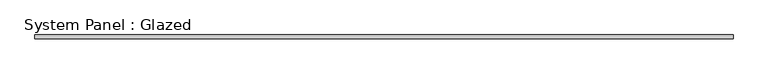
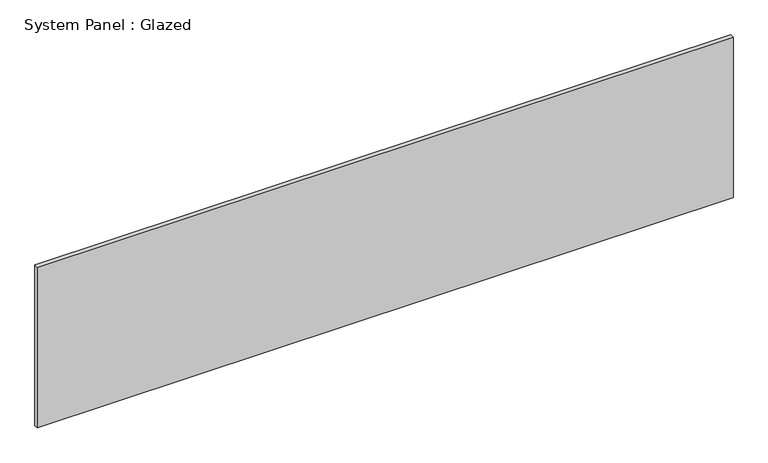
"""IFC4 building model written with IfcOpenShell, lengths in millimetres: plate geometry, System Panel : Glazed."""

from ifc_helpers import new_model, si_unit, origin, origin_with_axes, place, context, project, spatial, polyline, outline, extrude, source, transform, mapped, element, save


def system_panel_glazed_eef57662(model_context):
    return source(origin(), model_context, "Body", "SweptSolid", [
        extrude(outline(polyline([(2364.8485476, 19.05), (-2364.8485476, 19.05), (-2364.8485476, 44.45), (2364.8485476, 44.45), (2364.8485476, 19.05)])), origin_with_axes(), (0.0, 0.0, 1.0), 1155.7),
    ])


if __name__ == "__main__":
    model = new_model("IFC4")
    model_context = context("Model", 3, world=origin())
    ifc_project = project(units=[si_unit("LENGTHUNIT", "METRE", prefix="MILLI")], contexts=[model_context])
    site = spatial("IfcSite", under=ifc_project)
    building = spatial("IfcBuilding", under=site)
    placement = place(None, origin())
    system_panel_glazed_shape = system_panel_glazed_eef57662(model_context)
    element("IfcPlate", 1, ObjectType="System Panel : Glazed", at=placement, inside=building, context=model_context, shape_type="MappedRepresentation", body=[
        mapped(system_panel_glazed_shape, transform((0.0, 0.0, 0.0), x_axis=(1.0, 0.0, 0.0), y_axis=(0.0, 1.0, 0.0), z_axis=(0.0, 0.0, 1.0))),
    ])
    save(model, "model.ifc")

# Revit data of these elements
# Type "System Panel : Glazed"
#   Construction Type Id = "GSP4R"
#   Analytic Construction = "1/8 in Pilkington single glazing"
#   Visual Light Transmittance = 0.9
#   Solar Heat Gain Coefficient = 0.86
#   Heat Transfer Coefficient (U) = 1.18115 BTU/(h·ft²·°F)
# Element 1 (IfcPlate, "System Panel : Glazed")
#   Materials on its faces: "Glass"
# Materials
#   "Glass": class "Glass", colour RGB 0 128 192, transparency 0.75, Description = "Soda Lime Glass", Cost = 0
